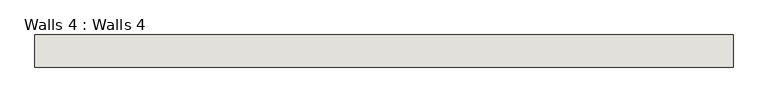
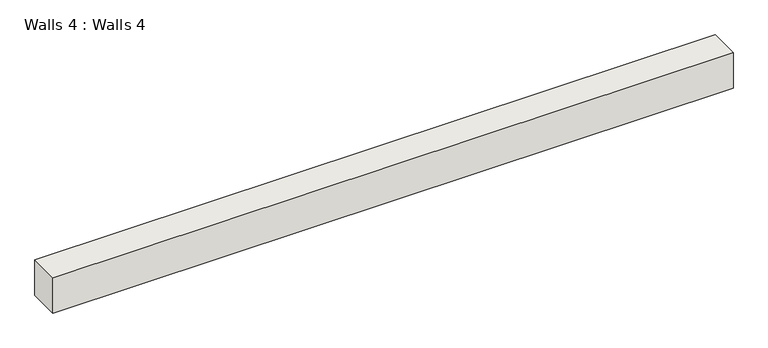
"""IFC4 building model written with IfcOpenShell, lengths in millimetres: wall geometry, Walls 4 : Walls 4."""

from ifc_helpers import new_model, si_unit, frame, origin, place, context, project, spatial, polyline, outline, extrude, source, transform, mapped, element, save


def walls_4_walls_4_4fd3bbeb(model_context):
    return source(origin(), model_context, "Body", "SweptSolid", [
        extrude(outline(polyline([(258.2694807, -3933.6430739), (-5897.2145744, -3933.6430739), (-5897.2145744, -3650.2259649), (258.2694807, -3650.2259649), (258.2694807, -3933.6430739)])), frame((0.0, 0.0, 6533.3350967), z_axis=(0.0, 0.0, 1.0), x_axis=(1.0, 0.0, 0.0)), (0.0, 0.0, 1.0), 338.9572127),
    ])


if __name__ == "__main__":
    model = new_model("IFC4")
    model_context = context("Model", 3, world=origin())
    ifc_project = project(units=[si_unit("LENGTHUNIT", "METRE", prefix="MILLI")], contexts=[model_context])
    site = spatial("IfcSite", under=ifc_project)
    building = spatial("IfcBuilding", under=site)
    placement = place(None, origin())
    walls_4_walls_4_shape = walls_4_walls_4_4fd3bbeb(model_context)
    element("IfcWall", 1, ObjectType="Walls 4 : Walls 4", at=placement, inside=building, context=model_context, shape_type="MappedRepresentation", body=[
        mapped(walls_4_walls_4_shape, transform((0.0, 0.0, 0.0), x_axis=(1.0, 0.0, 0.0), y_axis=(0.0, 1.0, 0.0), z_axis=(0.0, 0.0, 1.0))),
    ])
    save(model, "model.ifc")

# Revit data of these elements
# Element 1 (IfcWall, "Walls 4 : Walls 4")
#   Materials on its faces: "Default Wall"
# Materials
#   "Default Wall": colour RGB 128 128 128, transparency 0
